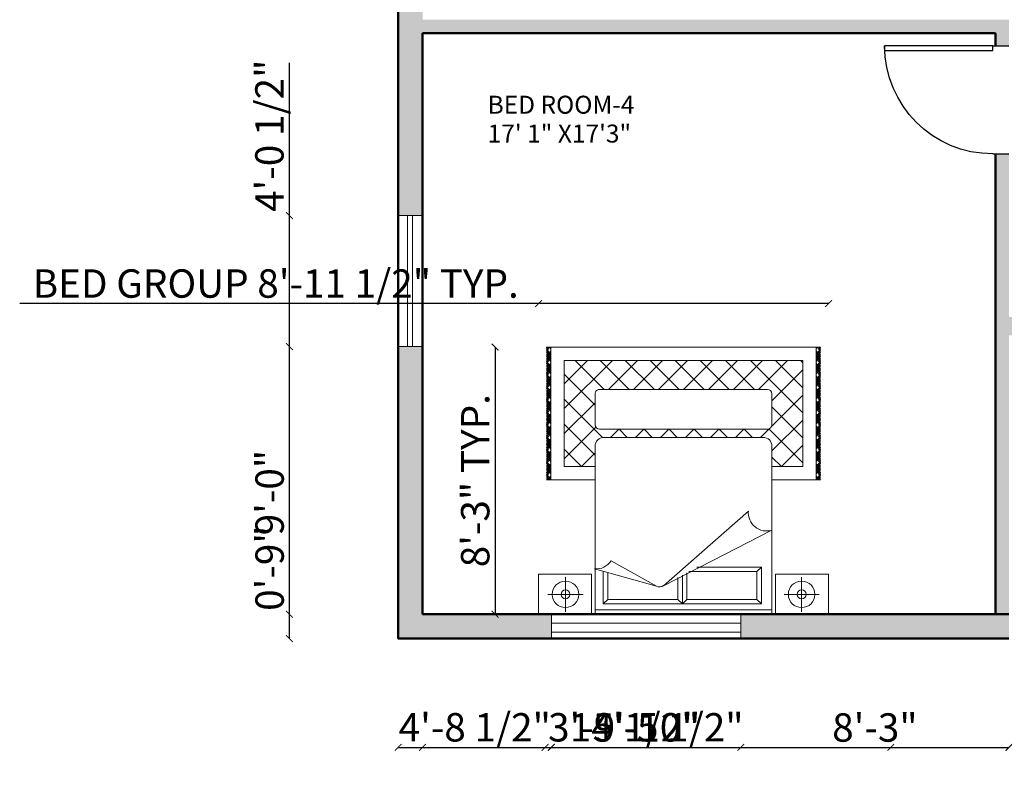
# Model space of a CAD drawing. Units: inches. Extents: x 1549 to 2410, y 1378 to 2139.
# Tile 1 of 6: x 1549 to 1913, y 1378 to 1657. Entities that reach past the tile are written whole.
import ezdxf

# ---------------------------------------------------------------- set-up
doc = ezdxf.new("R2010")
doc.units = ezdxf.units.IN
for name, color, linetype, lineweight in [('A-ANNO-DIMS', 2, 'Continuous', 18), ('A-AREA-IDEN', 7, 'Continuous', 18), ('A-DOOR', 4, 'Continuous', 25), ('A-FURN', 8, 'Continuous', 18), ('A-WALL', 7, 'Continuous', 50), ('WINDOW', 2, 'Continuous', 18)]:
    doc.layers.add(name, color=color, linetype=linetype, lineweight=lineweight)
doc.layers.add('A-WALL-PATT', color=18, linetype='Continuous', lineweight=13, true_color=0x000000)
doc.styles.get("Standard").update_dxf_attribs({"font": 'arial.ttf'})
doc.dimstyles.new('ISO-25', dxfattribs={"dimtxt": 10.5, "dimasz": 2.5, "dimexe": 1.25, "dimexo": 0.625, "dimtad": 1, "dimdec": 0, "dimlunit": 4, "dimtxsty": 'Standard', "dimblk": 'ARCHTICK', "dimcen": 2.5, "dimse1": 1, "dimse2": 1, "dimclrd": 1, "dimclrt": 3, "dimadec": 0, "dimazin": 0, "dimtfac": 1, "dimtdec": 0, "dimtmove": 0, "dimatfit": 3, "dimfxl": 1, "dimarcsym": 0})

# ---------------------------------------------------------------- blocks, each defined once
blk = doc.blocks.new('*U3')
for p, q in [((0, 0), (0, -6)), ((40, 0), (40, -6))]:
    blk.add_line(p, q)
blk.add_lwpolyline([(0, 0), (0, 40), (1.75, 40), (1.75, 0)], close=True)
blk.add_arc((0, 0), 40, 0, 90)
blk = doc.blocks.new('A$C4CB008C5')
for p, q in [((0, 3.019), (0.6, 3.019)), ((0, 2.569), (0, 3.019)), ((0.6, 3.019), (0.6, 2.569)), ((0.64, 1.121), (0.64, 3.021)), ((0.64, 3.021), (2.64, 3.021)), ((2.64, 3.021), (2.64, 1.121)), ((3.279, 3.019), (2.679, 3.019)), ((2.679, 3.019), (2.679, 2.569)), ((3.279, 2.569), (3.279, 3.019)), ((0.304, 2.6), (0.304, 2.992)), ((0.64, 2.971), (2.64, 2.971)), ((0.759, 2.905), (2.547, 2.905)), ((0.759, 2.489), (0.759, 2.905)), ((0.759, 2.905), (0.809, 2.855)), ((1.603, 2.855), (1.653, 2.905)), ((1.653, 2.905), (1.653, 2.579)), ((1.653, 2.905), (1.703, 2.855)), ((2.497, 2.855), (2.547, 2.905)), ((2.547, 2.905), (2.547, 2.54)), ((2.975, 2.6), (2.975, 2.992)), ((0.106, 2.796), (0.503, 2.796)), ((0.809, 2.855), (1.603, 2.855)), ((0.809, 2.539), (0.809, 2.855)), ((1.603, 2.855), (1.603, 2.551)), ((1.703, 2.855), (1.703, 2.607)), ((1.703, 2.855), (2.497, 2.855)), ((2.497, 2.855), (2.497, 2.556)), ((3.174, 2.796), (2.776, 2.796)), ((0.64, 2.071), (1.866, 2.698)), ((0.906, 1.854), (1.866, 2.698)), ((1.946, 2.705), (2.646, 2.507)), ((1.946, 2.705), (2.46, 2.418)), ((0.6, 2.569), (0, 2.569)), ((2.679, 2.569), (3.279, 2.569)), ((0.809, 2.539), (0.759, 2.489)), ((1.49, 2.489), (0.759, 2.489)), ((1.58, 2.539), (0.809, 2.539)), ((0.907, 1.867), (0.919, 1.867)), ((0.09, 1.5), (0.64, 1.5)), ((0.09, 1.491), (0.099, 1.5)), ((0.09, 1.473), (0.116, 1.5)), ((0.09, 1.456), (0.134, 1.5)), ((0.09, 1.474), (0.09, 1.475)), ((0.09, 1.438), (0.126, 1.474)), ((0.117, 1.43), (0.09, 1.457)), ((0.14, 1.46), (0.108, 1.492)), ((0.14, 1.478), (0.118, 1.5)), ((0.14, 1.496), (0.135, 1.5)), ((0.14, 0), (0.14, 1.5)), ((2.64, 1.5), (3.19, 1.5)), ((3.14, 1.496), (3.144, 1.5)), ((3.14, 1.478), (3.162, 1.5)), ((3.14, 1.5), (3.14, 0)), ((3.14, 1.46), (3.171, 1.492)), ((3.19, 1.456), (3.145, 1.5)), ((3.19, 1.438), (3.154, 1.474)), ((3.162, 1.43), (3.19, 1.457)), ((3.19, 1.473), (3.163, 1.5)), ((3.19, 1.491), (3.181, 1.5)), ((3.189, 1.474), (3.19, 1.475)), ((0.14, 1.389), (0.09, 1.439)), ((0.09, 1.42), (0.099, 1.43)), ((0.14, 1.372), (0.09, 1.422)), ((0.09, 1.368), (0.14, 1.417)), ((0.14, 1.354), (0.09, 1.404)), ((0.09, 1.35), (0.14, 1.4)), ((0.14, 1.336), (0.09, 1.386)), ((0.09, 1.332), (0.14, 1.382)), ((0.09, 1.314), (0.14, 1.364)), ((0.14, 1.319), (0.108, 1.35)), ((0.117, 1.412), (0.14, 1.435)), ((0.14, 1.442), (0.135, 1.448)), ((0.29, 1.108), (0.532, 1.35)), ((0.29, 0.15), (0.29, 1.35)), ((0.29, 1.35), (0.64, 1.35)), ((0.64, 1.243), (0.533, 1.35)), ((2.64, 1.195), (2.795, 1.35)), ((2.64, 1.35), (2.99, 1.35)), ((2.99, 1.156), (2.795, 1.35)), ((2.99, 1.35), (2.99, 0.15)), ((3.14, 1.442), (3.145, 1.448)), ((3.14, 1.389), (3.19, 1.439)), ((3.162, 1.412), (3.14, 1.435)), ((3.14, 1.372), (3.19, 1.422)), ((3.189, 1.368), (3.14, 1.417)), ((3.14, 1.354), (3.19, 1.404)), ((3.19, 1.35), (3.14, 1.4)), ((3.14, 1.336), (3.19, 1.386)), ((3.19, 1.332), (3.14, 1.382)), ((3.19, 1.314), (3.14, 1.364)), ((3.14, 1.319), (3.171, 1.35)), ((3.19, 1.42), (3.18, 1.43)), ((0.09, 1.297), (0.126, 1.333)), ((0.09, 1.333), (0.09, 1.333)), ((0.117, 1.288), (0.09, 1.316)), ((0.14, 1.248), (0.09, 1.298)), ((0.09, 1.279), (0.099, 1.288)), ((0.14, 1.23), (0.09, 1.28)), ((0.09, 1.227), (0.14, 1.276)), ((0.14, 1.213), (0.09, 1.263)), ((0.09, 1.208), (0.14, 1.258)), ((0.14, 1.195), (0.09, 1.245)), ((0.09, 1.19), (0.14, 1.24)), ((0.117, 1.271), (0.14, 1.294)), ((0.14, 1.301), (0.135, 1.306)), ((0.674, 0.926), (0.29, 1.31)), ((2.632, 0.904), (2.99, 1.262)), ((3.14, 1.301), (3.145, 1.306)), ((3.14, 1.248), (3.19, 1.298)), ((3.162, 1.271), (3.14, 1.294)), ((3.14, 1.23), (3.19, 1.28)), ((3.189, 1.227), (3.14, 1.276)), ((3.14, 1.213), (3.19, 1.263)), ((3.19, 1.208), (3.14, 1.258)), ((3.14, 1.195), (3.19, 1.245)), ((3.19, 1.19), (3.14, 1.24)), ((3.19, 1.297), (3.154, 1.333)), ((3.162, 1.288), (3.19, 1.316)), ((3.19, 1.279), (3.18, 1.288)), ((3.189, 1.333), (3.19, 1.333)), ((0.09, 1.173), (0.14, 1.223)), ((0.09, 1.191), (0.09, 1.192)), ((0.09, 1.155), (0.126, 1.191)), ((0.117, 1.147), (0.09, 1.174)), ((0.14, 1.107), (0.09, 1.157)), ((0.09, 1.137), (0.099, 1.147)), ((0.14, 1.089), (0.09, 1.139)), ((0.09, 1.085), (0.14, 1.134)), ((0.14, 1.071), (0.09, 1.121)), ((0.09, 1.067), (0.14, 1.117)), ((0.14, 1.177), (0.108, 1.209)), ((0.117, 1.129), (0.14, 1.152)), ((0.14, 1.16), (0.135, 1.165)), ((0.29, 0.825), (0.64, 1.175)), ((2.99, 0.873), (2.64, 1.223)), ((3.19, 1.173), (3.14, 1.223)), ((3.14, 1.177), (3.171, 1.209)), ((3.14, 1.16), (3.145, 1.165)), ((3.14, 1.107), (3.19, 1.157)), ((3.162, 1.129), (3.14, 1.152)), ((3.14, 1.089), (3.19, 1.139)), ((3.189, 1.085), (3.14, 1.134)), ((3.14, 1.071), (3.19, 1.121)), ((3.19, 1.067), (3.14, 1.117)), ((3.19, 1.155), (3.154, 1.191)), ((3.162, 1.147), (3.19, 1.174)), ((3.19, 1.137), (3.18, 1.147)), ((3.189, 1.191), (3.19, 1.192)), ((0.14, 1.054), (0.09, 1.104)), ((0.09, 1.049), (0.14, 1.099)), ((0.09, 1.031), (0.14, 1.081)), ((0.09, 1.05), (0.09, 1.051)), ((0.09, 1.014), (0.126, 1.05)), ((0.117, 1.006), (0.09, 1.033)), ((0.14, 0.965), (0.09, 1.015)), ((0.09, 0.996), (0.099, 1.006)), ((0.14, 1.036), (0.108, 1.067)), ((0.117, 0.988), (0.14, 1.011)), ((0.14, 1.018), (0.135, 1.023)), ((0.64, 0.677), (0.29, 1.027)), ((0.673, 0.925), (0.769, 1.021)), ((2.54, 1.021), (0.74, 1.021)), ((0.955, 0.928), (0.861, 1.021)), ((0.959, 0.928), (1.052, 1.021)), ((1.238, 0.928), (1.144, 1.021)), ((1.241, 0.928), (1.335, 1.021)), ((1.52, 0.928), (1.427, 1.021)), ((1.524, 0.928), (1.618, 1.021)), ((1.803, 0.928), (1.71, 1.021)), ((1.807, 0.928), (1.9, 1.021)), ((2.086, 0.928), (1.993, 1.021)), ((2.09, 0.928), (2.183, 1.021)), ((2.369, 0.928), (2.276, 1.021)), ((2.373, 0.928), (2.466, 1.021)), ((2.99, 0.59), (2.557, 1.023)), ((3.14, 1.054), (3.19, 1.104)), ((3.19, 1.049), (3.14, 1.099)), ((3.19, 1.031), (3.14, 1.081)), ((3.14, 1.036), (3.171, 1.067)), ((3.14, 1.018), (3.145, 1.023)), ((3.14, 0.965), (3.19, 1.015)), ((3.162, 0.988), (3.14, 1.011)), ((3.19, 1.014), (3.154, 1.05)), ((3.162, 1.006), (3.19, 1.033)), ((3.19, 0.996), (3.18, 1.006)), ((3.189, 1.05), (3.19, 1.051)), ((0.14, 0.948), (0.09, 0.998)), ((0.09, 0.944), (0.14, 0.993)), ((0.14, 0.93), (0.09, 0.98)), ((0.09, 0.925), (0.14, 0.975)), ((0.14, 0.912), (0.09, 0.962)), ((0.09, 0.908), (0.14, 0.958)), ((0.09, 0.89), (0.14, 0.94)), ((0.09, 0.908), (0.09, 0.909)), ((0.09, 0.872), (0.126, 0.908)), ((0.117, 0.864), (0.09, 0.891)), ((0.14, 0.894), (0.108, 0.926)), ((0.29, 0.542), (0.643, 0.895)), ((0.69, 0.928), (2.59, 0.928)), ((2.64, 0.629), (2.99, 0.979)), ((3.14, 0.948), (3.19, 0.998)), ((3.189, 0.944), (3.14, 0.993)), ((3.14, 0.93), (3.19, 0.98)), ((3.19, 0.925), (3.14, 0.975)), ((3.14, 0.912), (3.19, 0.962)), ((3.19, 0.908), (3.14, 0.958)), ((3.19, 0.89), (3.14, 0.94)), ((3.14, 0.894), (3.171, 0.926)), ((3.19, 0.872), (3.154, 0.908)), ((3.162, 0.864), (3.19, 0.891)), ((3.189, 0.908), (3.19, 0.909)), ((0.14, 0.824), (0.09, 0.874)), ((0.09, 0.855), (0.099, 0.864)), ((0.14, 0.806), (0.09, 0.856)), ((0.09, 0.802), (0.14, 0.852)), ((0.14, 0.788), (0.09, 0.838)), ((0.09, 0.784), (0.14, 0.834)), ((0.14, 0.771), (0.09, 0.821)), ((0.09, 0.766), (0.14, 0.816)), ((0.09, 0.749), (0.14, 0.799)), ((0.14, 0.753), (0.108, 0.785)), ((0.117, 0.847), (0.14, 0.869)), ((0.14, 0.877), (0.135, 0.882)), ((0.64, 0.878), (0.64, 0.528)), ((2.64, 0.878), (2.64, 0.528)), ((3.14, 0.877), (3.145, 0.882)), ((3.14, 0.824), (3.19, 0.874)), ((3.162, 0.847), (3.14, 0.869)), ((3.14, 0.806), (3.19, 0.856)), ((3.189, 0.802), (3.14, 0.852)), ((3.14, 0.788), (3.19, 0.838)), ((3.19, 0.784), (3.14, 0.834)), ((3.14, 0.771), (3.19, 0.821)), ((3.19, 0.766), (3.14, 0.816)), ((3.19, 0.749), (3.14, 0.799)), ((3.14, 0.753), (3.171, 0.785)), ((3.19, 0.855), (3.18, 0.864)), ((0.09, 0.767), (0.09, 0.768)), ((0.09, 0.731), (0.126, 0.767)), ((0.117, 0.723), (0.09, 0.75)), ((0.14, 0.682), (0.09, 0.732)), ((0.09, 0.713), (0.099, 0.723)), ((0.14, 0.665), (0.09, 0.715)), ((0.09, 0.661), (0.14, 0.71)), ((0.14, 0.647), (0.09, 0.697)), ((0.09, 0.642), (0.14, 0.692)), ((0.14, 0.629), (0.09, 0.679)), ((0.09, 0.625), (0.14, 0.675)), ((0.117, 0.705), (0.14, 0.728)), ((0.14, 0.735), (0.135, 0.74)), ((0.884, 0.15), (0.29, 0.744)), ((2.443, 0.15), (2.99, 0.696)), ((3.14, 0.735), (3.145, 0.74)), ((3.14, 0.682), (3.19, 0.732)), ((3.162, 0.705), (3.14, 0.728)), ((3.14, 0.665), (3.19, 0.715)), ((3.189, 0.661), (3.14, 0.71)), ((3.14, 0.647), (3.19, 0.697)), ((3.19, 0.642), (3.14, 0.692)), ((3.14, 0.629), (3.19, 0.679)), ((3.19, 0.625), (3.14, 0.675)), ((3.19, 0.731), (3.154, 0.767)), ((3.162, 0.723), (3.19, 0.75)), ((3.19, 0.713), (3.18, 0.723)), ((3.189, 0.767), (3.19, 0.768)), ((0.09, 0.607), (0.14, 0.657)), ((0.09, 0.589), (0.126, 0.626)), ((0.09, 0.626), (0.09, 0.626)), ((0.117, 0.581), (0.09, 0.609)), ((0.14, 0.541), (0.09, 0.591)), ((0.09, 0.572), (0.099, 0.581)), ((0.14, 0.523), (0.09, 0.573)), ((0.09, 0.519), (0.14, 0.569)), ((0.14, 0.612), (0.108, 0.643)), ((0.117, 0.564), (0.14, 0.586)), ((0.14, 0.594), (0.135, 0.599)), ((0.29, 0.259), (0.64, 0.609)), ((2.99, 0.307), (2.64, 0.657)), ((3.19, 0.607), (3.14, 0.657)), ((3.14, 0.612), (3.171, 0.643)), ((3.14, 0.594), (3.145, 0.599)), ((3.14, 0.541), (3.19, 0.591)), ((3.162, 0.564), (3.14, 0.586)), ((3.14, 0.523), (3.19, 0.573)), ((3.189, 0.519), (3.14, 0.569)), ((3.19, 0.589), (3.154, 0.626)), ((3.162, 0.581), (3.19, 0.609)), ((3.19, 0.572), (3.18, 0.581)), ((3.189, 0.626), (3.19, 0.626)), ((0.14, 0.506), (0.09, 0.556)), ((0.09, 0.501), (0.14, 0.551)), ((0.14, 0.488), (0.09, 0.538)), ((0.09, 0.483), (0.14, 0.533)), ((0.09, 0.466), (0.14, 0.516)), ((0.09, 0.484), (0.09, 0.485)), ((0.09, 0.448), (0.126, 0.484)), ((0.117, 0.44), (0.09, 0.467)), ((0.14, 0.399), (0.09, 0.449)), ((0.14, 0.47), (0.108, 0.502)), ((0.14, 0.453), (0.135, 0.458)), ((0.601, 0.15), (0.29, 0.462)), ((0.463, 0.15), (0.791, 0.478)), ((0.69, 0.478), (2.59, 0.478)), ((0.746, 0.15), (1.074, 0.478)), ((1.167, 0.15), (0.839, 0.478)), ((1.029, 0.15), (1.357, 0.478)), ((1.45, 0.15), (1.122, 0.478)), ((1.312, 0.15), (1.64, 0.478)), ((1.733, 0.15), (1.405, 0.478)), ((1.595, 0.15), (1.923, 0.478)), ((2.016, 0.15), (1.688, 0.478)), ((1.878, 0.15), (2.206, 0.478)), ((2.298, 0.15), (1.97, 0.478)), ((2.16, 0.15), (2.488, 0.478)), ((2.581, 0.15), (2.253, 0.478)), ((2.864, 0.15), (2.536, 0.478)), ((3.14, 0.506), (3.19, 0.556)), ((3.19, 0.501), (3.14, 0.551)), ((3.14, 0.488), (3.19, 0.538)), ((3.19, 0.483), (3.14, 0.533)), ((3.19, 0.466), (3.14, 0.516)), ((3.14, 0.47), (3.171, 0.502)), ((3.14, 0.453), (3.145, 0.458)), ((3.14, 0.399), (3.19, 0.449)), ((3.19, 0.448), (3.154, 0.484)), ((3.162, 0.44), (3.19, 0.467)), ((3.189, 0.484), (3.19, 0.485)), ((0.09, 0.43), (0.099, 0.44)), ((0.14, 0.382), (0.09, 0.432)), ((0.09, 0.378), (0.14, 0.427)), ((0.14, 0.364), (0.09, 0.414)), ((0.09, 0.36), (0.14, 0.41)), ((0.14, 0.346), (0.09, 0.396)), ((0.09, 0.342), (0.14, 0.392)), ((0.09, 0.324), (0.14, 0.374)), ((0.09, 0.307), (0.126, 0.343)), ((0.09, 0.343), (0.09, 0.343)), ((0.14, 0.329), (0.108, 0.36)), ((0.117, 0.422), (0.14, 0.445)), ((2.726, 0.15), (2.99, 0.414)), ((3.162, 0.422), (3.14, 0.445)), ((3.14, 0.382), (3.19, 0.432)), ((3.189, 0.378), (3.14, 0.427)), ((3.14, 0.364), (3.19, 0.414)), ((3.19, 0.36), (3.14, 0.41)), ((3.14, 0.346), (3.19, 0.396)), ((3.19, 0.342), (3.14, 0.392)), ((3.19, 0.324), (3.14, 0.374)), ((3.14, 0.329), (3.171, 0.36)), ((3.19, 0.307), (3.154, 0.343)), ((3.19, 0.43), (3.18, 0.44)), ((3.189, 0.343), (3.19, 0.343)), ((0.117, 0.299), (0.09, 0.326)), ((0.14, 0.258), (0.09, 0.308)), ((0.09, 0.289), (0.099, 0.299)), ((0.14, 0.24), (0.09, 0.29)), ((0.09, 0.237), (0.14, 0.286)), ((0.14, 0.223), (0.09, 0.273)), ((0.09, 0.218), (0.14, 0.268)), ((0.14, 0.205), (0.09, 0.255)), ((0.09, 0.201), (0.14, 0.251)), ((0.09, 0.183), (0.14, 0.233)), ((0.117, 0.281), (0.14, 0.304)), ((0.14, 0.311), (0.135, 0.316)), ((3.14, 0.311), (3.145, 0.316)), ((3.14, 0.258), (3.19, 0.308)), ((3.162, 0.281), (3.14, 0.304)), ((3.14, 0.24), (3.19, 0.29)), ((3.189, 0.237), (3.14, 0.286)), ((3.14, 0.223), (3.19, 0.273)), ((3.19, 0.218), (3.14, 0.268)), ((3.14, 0.205), (3.19, 0.255)), ((3.19, 0.201), (3.14, 0.251)), ((3.19, 0.183), (3.14, 0.233)), ((3.162, 0.299), (3.19, 0.326)), ((3.19, 0.289), (3.18, 0.299)), ((0.09, 0.201), (0.09, 0.202)), ((0.09, 0.165), (0.126, 0.201)), ((0.117, 0.157), (0.09, 0.184)), ((0.14, 0.117), (0.09, 0.167)), ((0.09, 0.148), (0.099, 0.157)), ((0.14, 0.099), (0.09, 0.149)), ((0.09, 0.095), (0.14, 0.144)), ((0.14, 0.081), (0.09, 0.131)), ((0.09, 0.077), (0.14, 0.127)), ((0.14, 0.064), (0.09, 0.114)), ((0.14, 0.187), (0.108, 0.219)), ((0.117, 0.139), (0.14, 0.162)), ((0.14, 0.17), (0.135, 0.175)), ((0.318, 0.15), (0.29, 0.179)), ((2.99, 0.15), (0.29, 0.15)), ((3.14, 0.187), (3.171, 0.219)), ((3.14, 0.17), (3.145, 0.175)), ((3.14, 0.117), (3.19, 0.167)), ((3.162, 0.139), (3.14, 0.162)), ((3.14, 0.099), (3.19, 0.149)), ((3.189, 0.095), (3.14, 0.144)), ((3.14, 0.081), (3.19, 0.131)), ((3.19, 0.077), (3.14, 0.127)), ((3.14, 0.064), (3.19, 0.114)), ((3.19, 0.165), (3.154, 0.201)), ((3.162, 0.157), (3.19, 0.184)), ((3.19, 0.148), (3.18, 0.157)), ((3.189, 0.201), (3.19, 0.202)), ((0.09, 0.059), (0.14, 0.109)), ((0.09, 0.041), (0.14, 0.091)), ((0.09, 0.06), (0.09, 0.061)), ((0.09, 0.024), (0.126, 0.06)), ((0.117, 0.016), (0.09, 0.043)), ((0.115, 0), (0.09, 0.025)), ((0.09, 0.006), (0.099, 0.016)), ((0.097, 0), (0.09, 0.008)), ((0.14, 0.046), (0.108, 0.078)), ((0.119, 0), (0.14, 0.021)), ((0.14, 0.028), (0.135, 0.033)), ((0.137, 0), (0.14, 0.003)), ((3.19, 0.059), (3.14, 0.109)), ((3.19, 0.041), (3.14, 0.091)), ((3.14, 0.046), (3.171, 0.078)), ((3.14, 0.028), (3.145, 0.033)), ((3.16, 0), (3.14, 0.021)), ((3.143, 0), (3.14, 0.003)), ((3.19, 0.024), (3.154, 0.06)), ((3.162, 0.016), (3.19, 0.043)), ((3.164, 0), (3.19, 0.025)), ((3.19, 0.006), (3.18, 0.016)), ((3.182, 0), (3.19, 0.008)), ((3.189, 0.06), (3.19, 0.061)), ((0.09, 0), (3.19, 0))]:
    blk.add_line(p, q)
for centre, radius in [((0.304, 2.796), 0.15), ((2.975, 2.796), 0.15), ((0.304, 2.796), 0.05), ((2.975, 2.796), 0.05)]:
    blk.add_circle(centre, radius)
for centre, radius, start, end in [((1.915, 2.61), 0.1, 71.7215, 119.0799), ((2.626, 2.31), 0.198, 84.1725, 146.9889), ((0.7, 1.873), 0.207, 354.6422, 106.9775), ((0.74, 1.121), 0.1, 180, 270), ((2.54, 1.121), 0.1, 270, 0), ((0.69, 0.878), 0.05, 90, 180), ((2.59, 0.878), 0.05, 0, 90), ((0.69, 0.528), 0.05, 180, 270), ((2.59, 0.528), 0.05, 270, 0)]:
    blk.add_arc(centre, radius, start, end)
blk = doc.blocks.new('_ArchTick')
at = {"color": 0, "linetype": 'ByBlock', "const_width": 0.15}
blk.add_lwpolyline([(-0.5, -0.5), (0.5, 0.5)], dxfattribs=at)
blk = doc.blocks.new('*D15')
at = {"layer": 'A-ANNO-DIMS', "color": 1, "lineweight": -2, "transparency": 16777216}
for p, q in [((1740.55, 1551.97), (1548.54, 1551.97)), ((1847.85, 1551.97), (1740.55, 1551.97))]:
    blk.add_line(p, q, dxfattribs=at)
at = {"layer": 'Defpoints', "color": 0, "transparency": 16777216}
for p in [(1740.55, 1551.97), (1740.55, 1535.87), (1847.85, 1535.87)]:
    blk.add_point(p, dxfattribs=at)
at = {"layer": 'A-ANNO-DIMS', "color": 1, "lineweight": -2, "transparency": 16777216, "xscale": 2.5, "yscale": 2.5, "zscale": 2.5, "rotation": 180}
blk.add_blockref('_ArchTick', (1740.55, 1551.97), dxfattribs=at)
at = {"layer": 'A-ANNO-DIMS', "color": 1, "lineweight": -2, "transparency": 16777216, "xscale": 2.5, "yscale": 2.5, "zscale": 2.5}
blk.add_blockref('_ArchTick', (1847.85, 1551.97), dxfattribs=at)
at = {"layer": 'A-ANNO-DIMS', "color": 3, "transparency": 16777216, "insert": (1643.29, 1558.03), "char_height": 10.5, "attachment_point": 5}
blk.add_mtext('BED GROUP 8\'-11 1/2" TYP.', dxfattribs=at)
blk = doc.blocks.new('*D16')
at = {"layer": 'A-ANNO-DIMS', "color": 1, "lineweight": -2, "transparency": 16777216}
blk.add_line((1724.45, 1535.87), (1724.45, 1437.01), dxfattribs=at)
at = {"layer": 'Defpoints', "color": 0, "transparency": 16777216}
for p in [(1740.55, 1535.87), (1724.45, 1437.01), (1740.55, 1437.01)]:
    blk.add_point(p, dxfattribs=at)
at = {"layer": 'A-ANNO-DIMS', "color": 1, "lineweight": -2, "transparency": 16777216, "xscale": 2.5, "yscale": 2.5, "zscale": 2.5}
for p, rotation in [((1724.45, 1535.87), 90), ((1724.45, 1437.01), 270)]:
    blk.add_blockref('_ArchTick', p, dxfattribs=dict(at, rotation=rotation))
at = {"layer": 'A-ANNO-DIMS', "color": 3, "transparency": 16777216, "insert": (1718.46, 1486.44), "char_height": 10.5, "attachment_point": 5, "rotation": 90}
blk.add_mtext('8\'-3" TYP.', dxfattribs=at)
blk = doc.blocks.new('*D27')
at = {"layer": 'A-ANNO-DIMS', "color": 1, "lineweight": -2, "transparency": 16777216}
blk.add_line((1688.62, 1387.76), (1745.28, 1387.76), dxfattribs=at)
at = {"layer": 'Defpoints', "color": 0, "transparency": 16777216}
for p in [(1688.62, 1428.01), (1745.28, 1428.01), (1745.28, 1387.76)]:
    blk.add_point(p, dxfattribs=at)
at = {"layer": 'A-ANNO-DIMS', "color": 1, "lineweight": -2, "transparency": 16777216, "xscale": 2.5, "yscale": 2.5, "zscale": 2.5, "rotation": 180}
blk.add_blockref('_ArchTick', (1688.62, 1387.76), dxfattribs=at)
at = {"layer": 'A-ANNO-DIMS', "color": 1, "lineweight": -2, "transparency": 16777216, "xscale": 2.5, "yscale": 2.5, "zscale": 2.5}
blk.add_blockref('_ArchTick', (1745.28, 1387.76), dxfattribs=at)
at = {"layer": 'A-ANNO-DIMS', "color": 3, "transparency": 16777216, "insert": (1716.95, 1393.82), "char_height": 10.5, "attachment_point": 5}
blk.add_mtext('4\'-8 1/2"', dxfattribs=at)
blk = doc.blocks.new('*D28')
at = {"layer": 'A-ANNO-DIMS', "color": 1, "lineweight": -2, "transparency": 16777216}
blk.add_line((1745.28, 1387.76), (1815.42, 1387.76), dxfattribs=at)
at = {"layer": 'Defpoints', "color": 0, "transparency": 16777216}
for p in [(1745.28, 1428.01), (1815.42, 1428.01), (1815.42, 1387.76)]:
    blk.add_point(p, dxfattribs=at)
at = {"layer": 'A-ANNO-DIMS', "color": 1, "lineweight": -2, "transparency": 16777216, "xscale": 2.5, "yscale": 2.5, "zscale": 2.5, "rotation": 180}
blk.add_blockref('_ArchTick', (1745.28, 1387.76), dxfattribs=at)
at = {"layer": 'A-ANNO-DIMS', "color": 1, "lineweight": -2, "transparency": 16777216, "xscale": 2.5, "yscale": 2.5, "zscale": 2.5}
blk.add_blockref('_ArchTick', (1815.42, 1387.76), dxfattribs=at)
at = {"layer": 'A-ANNO-DIMS', "color": 3, "transparency": 16777216, "insert": (1780.35, 1393.75), "char_height": 10.5, "attachment_point": 5}
blk.add_mtext('5\'-10"', dxfattribs=at)
blk = doc.blocks.new('*D29')
at = {"layer": 'A-ANNO-DIMS', "color": 1, "lineweight": -2, "transparency": 16777216}
blk.add_line((1815.42, 1387.76), (1914.62, 1387.76), dxfattribs=at)
at = {"layer": 'Defpoints', "color": 0, "transparency": 16777216}
for p in [(1815.42, 1428.01), (1914.62, 1428.01), (1914.62, 1387.76)]:
    blk.add_point(p, dxfattribs=at)
at = {"layer": 'A-ANNO-DIMS', "color": 1, "lineweight": -2, "transparency": 16777216, "xscale": 2.5, "yscale": 2.5, "zscale": 2.5, "rotation": 180}
blk.add_blockref('_ArchTick', (1815.42, 1387.76), dxfattribs=at)
at = {"layer": 'A-ANNO-DIMS', "color": 1, "lineweight": -2, "transparency": 16777216, "xscale": 2.5, "yscale": 2.5, "zscale": 2.5}
blk.add_blockref('_ArchTick', (1914.62, 1387.76), dxfattribs=at)
at = {"layer": 'A-ANNO-DIMS', "color": 3, "transparency": 16777216, "insert": (1865.02, 1393.75), "char_height": 10.5, "attachment_point": 5}
blk.add_mtext('8\'-3"', dxfattribs=at)
blk = doc.blocks.new('*D35')
at = {"layer": 'A-ANNO-DIMS', "color": 1, "lineweight": -2, "transparency": 16777216}
blk.add_line((1648.37, 1428.01), (1648.37, 1536.06), dxfattribs=at)
at = {"layer": 'Defpoints', "color": 0, "transparency": 16777216}
for p in [(1648.37, 1536.06), (1688.62, 1536.06), (1688.62, 1428.01)]:
    blk.add_point(p, dxfattribs=at)
at = {"layer": 'A-ANNO-DIMS', "color": 1, "lineweight": -2, "transparency": 16777216, "xscale": 2.5, "yscale": 2.5, "zscale": 2.5}
for p, rotation in [((1648.37, 1536.06), 90), ((1648.37, 1428.01), 270)]:
    blk.add_blockref('_ArchTick', p, dxfattribs=dict(at, rotation=rotation))
at = {"layer": 'A-ANNO-DIMS', "color": 3, "transparency": 16777216, "insert": (1642.38, 1482.04), "char_height": 10.5, "attachment_point": 5, "rotation": 90}
blk.add_mtext('9\'-0"', dxfattribs=at)
blk = doc.blocks.new('*D36')
at = {"layer": 'A-ANNO-DIMS', "color": 1, "lineweight": -2, "transparency": 16777216}
for p, q in [((1648.37, 1584.55), (1648.37, 1641.1)), ((1648.37, 1536.06), (1648.37, 1584.55))]:
    blk.add_line(p, q, dxfattribs=at)
at = {"layer": 'Defpoints', "color": 0, "transparency": 16777216}
for p in [(1648.37, 1584.55), (1688.62, 1584.55), (1688.62, 1536.06)]:
    blk.add_point(p, dxfattribs=at)
at = {"layer": 'A-ANNO-DIMS', "color": 1, "lineweight": -2, "transparency": 16777216, "xscale": 2.5, "yscale": 2.5, "zscale": 2.5}
for p, rotation in [((1648.37, 1584.55), 90), ((1648.37, 1536.06), 270)]:
    blk.add_blockref('_ArchTick', p, dxfattribs=dict(at, rotation=rotation))
at = {"layer": 'A-ANNO-DIMS', "color": 3, "transparency": 16777216, "insert": (1642.31, 1614.08), "char_height": 10.5, "attachment_point": 5, "rotation": 90}
blk.add_mtext('4\'-0 1/2"', dxfattribs=at)
blk = doc.blocks.new('*D55')
at = {"layer": 'A-ANNO-DIMS', "color": 1, "lineweight": -2, "transparency": 16777216}
for p, q in [((1648.37, 1437.01), (1648.37, 1468.68)), ((1648.37, 1428.01), (1648.37, 1437.01))]:
    blk.add_line(p, q, dxfattribs=at)
at = {"layer": 'Defpoints', "color": 0, "transparency": 16777216}
for p in [(1648.37, 1437.01), (1697.62, 1437.01), (1688.62, 1428.01)]:
    blk.add_point(p, dxfattribs=at)
at = {"layer": 'A-ANNO-DIMS', "color": 1, "lineweight": -2, "transparency": 16777216, "xscale": 2.5, "yscale": 2.5, "zscale": 2.5}
for p, rotation in [((1648.37, 1437.01), 90), ((1648.37, 1428.01), 270)]:
    blk.add_blockref('_ArchTick', p, dxfattribs=dict(at, rotation=rotation))
at = {"layer": 'A-ANNO-DIMS', "color": 3, "transparency": 16777216, "insert": (1642.38, 1454.1), "char_height": 10.5, "attachment_point": 5, "rotation": 90}
blk.add_mtext('0\'-9"', dxfattribs=at)
blk = doc.blocks.new('*D60')
at = {"layer": 'A-ANNO-DIMS', "color": 1, "lineweight": -2, "transparency": 16777216}
blk.add_line((2400.7, 1657.01), (2400.7, 1709.88), dxfattribs=at)
at = {"layer": 'Defpoints', "color": 0, "transparency": 16777216}
for p in [(1870.93, 1709.88), (2400.7, 1709.88), (1870.93, 1657.01)]:
    blk.add_point(p, dxfattribs=at)
at = {"layer": 'A-ANNO-DIMS', "color": 1, "lineweight": -2, "transparency": 16777216, "xscale": 2.5, "yscale": 2.5, "zscale": 2.5}
for p, rotation in [((2400.7, 1709.88), 90), ((2400.7, 1657.01), 270)]:
    blk.add_blockref('_ArchTick', p, dxfattribs=dict(at, rotation=rotation))
at = {"layer": 'A-ANNO-DIMS', "color": 3, "transparency": 16777216, "insert": (2394.74, 1683.45), "char_height": 10.5, "attachment_point": 5, "rotation": 90}
blk.add_mtext('4\'-5"', dxfattribs=at)
blk = doc.blocks.new('*D61')
at = {"layer": 'A-ANNO-DIMS', "color": 1, "lineweight": -2, "transparency": 16777216}
for p, q in [((1697.62, 1387.76), (1742.95, 1387.76)), ((1742.95, 1387.76), (1799.07, 1387.76))]:
    blk.add_line(p, q, dxfattribs=at)
at = {"layer": 'Defpoints', "color": 0, "transparency": 16777216}
for p in [(1697.62, 1764.95), (1742.95, 1764.95), (1742.95, 1387.76)]:
    blk.add_point(p, dxfattribs=at)
at = {"layer": 'A-ANNO-DIMS', "color": 1, "lineweight": -2, "transparency": 16777216, "xscale": 2.5, "yscale": 2.5, "zscale": 2.5, "rotation": 180}
blk.add_blockref('_ArchTick', (1697.62, 1387.76), dxfattribs=at)
at = {"layer": 'A-ANNO-DIMS', "color": 1, "lineweight": -2, "transparency": 16777216, "xscale": 2.5, "yscale": 2.5, "zscale": 2.5}
blk.add_blockref('_ArchTick', (1742.95, 1387.76), dxfattribs=at)
at = {"layer": 'A-ANNO-DIMS', "color": 3, "transparency": 16777216, "insert": (1772.26, 1393.82), "char_height": 10.5, "attachment_point": 5}
blk.add_mtext('3\'-9 1/2"', dxfattribs=at)
blk = doc.blocks.new('*D62')
at = {"layer": 'A-ANNO-DIMS', "color": 1, "lineweight": -2, "transparency": 16777216}
blk.add_line((1697.62, 1387.76), (1870.93, 1387.76), dxfattribs=at)
at = {"layer": 'Defpoints', "color": 0, "transparency": 16777216}
for p in [(1697.62, 1657.01), (1870.93, 1657.01), (1870.93, 1387.76)]:
    blk.add_point(p, dxfattribs=at)
at = {"layer": 'A-ANNO-DIMS', "color": 1, "lineweight": -2, "transparency": 16777216, "xscale": 2.5, "yscale": 2.5, "zscale": 2.5, "rotation": 180}
blk.add_blockref('_ArchTick', (1697.62, 1387.76), dxfattribs=at)
at = {"layer": 'A-ANNO-DIMS', "color": 1, "lineweight": -2, "transparency": 16777216, "xscale": 2.5, "yscale": 2.5, "zscale": 2.5}
blk.add_blockref('_ArchTick', (1870.93, 1387.76), dxfattribs=at)
at = {"layer": 'A-ANNO-DIMS', "color": 3, "transparency": 16777216, "insert": (1784.28, 1393.82), "char_height": 10.5, "attachment_point": 5}
blk.add_mtext('14\'-5 1/2"', dxfattribs=at)

msp = doc.modelspace()

# ---------------------------------------------------------------- hatches: boundary and pattern name
at = {"layer": 'A-WALL-PATT'}
h = msp.add_hatch(color=256, dxfattribs=at)
h.dxf.hatch_style = 1
h.paths.add_polyline_path([(1760, 2069.01), (1688.62, 2069.01), (1688.62, 2003.68), (1697.62, 2003.68), (1697.62, 2060.01), (1760, 2060.01)])
h.paths.add_polyline_path([(2309.62, 2069.01), (1807.68, 2069.01), (1807.68, 2060.01), (1909.62, 2060.01), (1909.62, 2040.27), (1914.62, 2040.27), (1914.62, 2060.01), (2082.62, 2060.01), (2082.62, 2043.41), (2087.62, 2043.41), (2087.62, 2060.01), (2300.62, 2060.01), (2300.62, 2006.22), (2309.62, 2006.22)])
h.paths.add_polyline_path([(1914.62, 1607.36), (1909.62, 1607.36), (1909.62, 1437.01), (1914.62, 1437.01)])
h.paths.add_polyline_path([(1697.62, 1536.06), (1688.62, 1536.06), (1688.62, 1428.01), (1745.28, 1428.01), (1745.28, 1437.01), (1697.62, 1437.01)])
h.paths.add_polyline_path([(2130.61, 1437.01), (2082.62, 1437.01), (2082.62, 1428.01), (2130.61, 1428.01)])
h.paths.add_polyline_path([(2309.62, 1544.51), (2302.25, 1544.51), (2302.25, 1524.81), (2300.62, 1524.81), (2300.62, 1523.51), (2302.17, 1523.51), (2302.17, 1503.88), (2300.62, 1503.88), (2300.62, 1437.01), (2193.34, 1437.01), (2193.34, 1428.01), (2309.62, 1428.01)])
h.paths.add_polyline_path([(2309.62, 1708.66), (2300.62, 1708.66), (2300.62, 1657.01), (2293.7, 1657.01), (2293.7, 1652.01), (2300.62, 1652.01), (2300.62, 1611.18), (2302.17, 1611.18), (2302.17, 1597.64), (2309.62, 1597.64)])
h.paths.add_polyline_path([(2309.62, 1777.38), (2300.62, 1777.38), (2300.62, 1737.9), (2309.62, 1737.9)])
h.paths.add_polyline_path([(2300.62, 1757.01), (2168.62, 1757.01), (2168.62, 1795.96), (2163.62, 1795.96), (2163.62, 1657.01), (2082.62, 1657.01), (2082.62, 1641.99), (2087.62, 1641.99), (2087.62, 1652.01), (2253.7, 1652.01), (2253.7, 1657.01), (2168.62, 1657.01), (2168.62, 1752.01), (2300.62, 1752.01)])
h.paths.add_polyline_path([(2309.62, 1957.79), (2300.62, 1957.79), (2300.62, 1935.33), (2300.62, 1824.93), (2309.62, 1824.93)])
h.paths.add_polyline_path([(2300.62, 1849.01), (2137.17, 1849.01), (2137.17, 1844.01), (2163.62, 1844.01), (2163.62, 1835.96), (2168.62, 1835.96), (2168.62, 1844.01), (2300.62, 1844.01)])
h.paths.add_polyline_path([(2211.06, 1800.23), (2261.76, 1800.23), (2261.76, 1810.41), (2211.06, 1810.41)], flags=9)
h.paths.add_polyline_path([(2211.1, 1811.05), (2239.18, 1811.05), (2239.18, 1821.02), (2211.1, 1821.02)], flags=9)
h.paths.add_polyline_path([(2187.84, 1718.73), (2233.38, 1718.73), (2233.38, 1728.91), (2187.84, 1728.91)], flags=25)
h.paths.add_polyline_path([(2187.88, 1729.56), (2215.96, 1729.56), (2215.96, 1739.52), (2187.88, 1739.52)], flags=25)
h.paths.add_polyline_path([(1720.01, 1609.74), (1775.87, 1609.74), (1775.87, 1619.93), (1720.01, 1619.93)], flags=9)
h.paths.add_polyline_path([(1719.99, 1620.4), (1782.23, 1620.4), (1782.23, 1630.72), (1719.99, 1630.72)], flags=9)
h.paths.add_polyline_path([(2092.97, 1541.04), (2148.83, 1541.04), (2148.83, 1551.23), (2092.97, 1551.23)], flags=9)
h.paths.add_polyline_path([(2092.94, 1551.69), (2155.19, 1551.69), (2155.19, 1562.02), (2092.94, 1562.02)], flags=9)
h.paths.add_polyline_path([(1759.73, 1747.67), (1815.59, 1747.67), (1815.59, 1757.85), (1759.73, 1757.85)], flags=9)
h.paths.add_polyline_path([(1759.71, 1758.32), (1790.48, 1758.32), (1790.48, 1768.63), (1759.71, 1768.63)], flags=9)
h.paths.add_polyline_path([(1940.79, 1793.43), (1996.65, 1793.43), (1996.65, 1803.61), (1940.79, 1803.61)], flags=9)
h.paths.add_polyline_path([(1940.77, 1804.08), (2006.11, 1804.08), (2006.11, 1814.4), (1940.77, 1814.4)], flags=9)
h.paths.add_polyline_path([(2094.62, 1963.23), (2150.43, 1963.23), (2150.43, 1973.25), (2094.62, 1973.25)], flags=9)
h.paths.add_polyline_path([(2094.57, 1973.75), (2156.81, 1973.75), (2156.81, 1984.07), (2094.57, 1984.07)], flags=9)
h.paths.add_polyline_path([(1943.36, 1930.19), (2000.28, 1930.19), (2000.28, 1940.37), (1943.36, 1940.37)], flags=9)
h.paths.add_polyline_path([(1943.34, 1940.85), (1987.53, 1940.85), (1987.53, 1951.15), (1943.34, 1951.15)], flags=9)
h.paths.add_polyline_path([(1803.94, 1971.5), (1857.22, 1971.5), (1857.22, 1981.68), (1803.94, 1981.68)], flags=9)
h.paths.add_polyline_path([(1803.92, 1982.16), (1866.16, 1982.16), (1866.16, 1992.47), (1803.92, 1992.47)], flags=9)
h = msp.add_hatch(color=256, dxfattribs=at)
h.dxf.hatch_style = 1
h.paths.add_polyline_path([(1697.62, 1844.01), (1688.62, 1844.01), (1688.62, 1657.01), (1697.62, 1657.01)])
h.paths.add_polyline_path([(1697.62, 1955.9), (1688.62, 1955.9), (1688.62, 1844.01), (1697.62, 1844.01), (1867.86, 1844.01), (1867.86, 1849.01), (1697.62, 1849.01)])
h.paths.add_polyline_path([(1697.62, 1652.01), (1909.62, 1652.01), (1909.62, 1647.36), (1914.62, 1647.36), (1914.62, 1657.01), (1697.62, 1657.01), (1688.62, 1657.01), (1688.62, 1584.55), (1697.62, 1584.55)])
h.paths.add_polyline_path([(2087.62, 1601.99), (2082.62, 1601.99), (2082.62, 1437.01), (2087.62, 1437.01)])
h.paths.add_polyline_path([(1981.52, 1547.01), (1914.62, 1547.01), (1914.62, 1540.24), (1981.52, 1540.24)])
h.paths.add_polyline_path([(2082.62, 1547.01), (2061.69, 1547.01), (2061.69, 1540.24), (2082.62, 1540.24)])
h = msp.add_hatch(color=256, dxfattribs=at)
h.dxf.hatch_style = 1
h.paths.add_polyline_path([(1914.62, 1437.01), (1815.42, 1437.01), (1815.42, 1428.01), (1914.62, 1428.01)])

# ---------------------------------------------------------------- linework, layer by layer
at = {"layer": 'A-WALL'}
for p, q in [((1697.62, 1437.01), (1697.62, 1652.01)), ((1697.62, 1652.01), (1909.62, 1652.01)), ((1909.62, 1647.36), (1909.62, 1652.01)), ((1909.62, 1437.01), (1909.62, 1607.36)), ((1914.62, 1437.01), (1697.62, 1437.01))]:
    msp.add_line(p, q, dxfattribs=at)
msp.add_lwpolyline([(1914.62, 1428.01), (1688.62, 1428.01), (1688.62, 2069.01), (2309.62, 2069.01), (2309.62, 1428.01), (2082.62, 1428.01)], dxfattribs=at)
at = {"layer": 'WINDOW'}
for p, q in [((1697.62, 1584.55), (1688.62, 1584.55)), ((1688.62, 1584.55), (1688.62, 1536.06)), ((1692.06, 1536.06), (1692.06, 1584.55)), ((1693.9, 1536.06), (1693.9, 1584.55)), ((1697.62, 1536.06), (1697.62, 1584.55)), ((1688.62, 1536.06), (1697.62, 1536.06)), ((1745.28, 1437.01), (1745.28, 1428.01)), ((1815.42, 1437.01), (1745.28, 1437.01)), ((1815.42, 1428.01), (1815.42, 1437.01)), ((1815.42, 1433.76), (1745.28, 1433.76)), ((1815.42, 1430.41), (1745.28, 1430.41)), ((1745.28, 1428.01), (1815.42, 1428.01))]:
    msp.add_line(p, q, dxfattribs=at)

# ---------------------------------------------------------------- block references
at = {"layer": 'A-DOOR', "xscale": -1, "rotation": 90}
msp.add_blockref('*U3', (1908.62, 1647.36), dxfattribs=at)
at = {"layer": 'A-FURN', "xscale": 32.72052747801291, "yscale": 32.72052747801291, "zscale": 32.72052747801291, "rotation": 180}
msp.add_blockref('A$C4CB008C5', (1847.85, 1535.87), dxfattribs=at)

# ---------------------------------------------------------------- texts
at = {"layer": 'A-AREA-IDEN'}
for s, height, p in [('BED ROOM-4', 6.645, (1721.71, 1622.23)), ('17\' 1" X17\'3"', 6.6455, (1721.71, 1611.56))]:
    msp.add_text(s, height=height, dxfattribs=at).set_placement(p)

# ---------------------------------------------------------------- dimensions: what is measured, and where the dimension line sits
at = {"layer": 'A-ANNO-DIMS'}
for base, p1, p2, picture, middle in [((1742.95, 1387.76), (1697.62, 1764.95), (1742.95, 1764.95), '*D61', (1772.26, 1393.82)), ((1870.93, 1387.76), (1697.62, 1657.01), (1870.93, 1657.01), '*D62', (1784.28, 1393.82)), ((1745.28, 1387.76), (1688.62, 1428.01), (1745.28, 1428.01), '*D27', (1716.95, 1393.82)), ((1815.42, 1387.76), (1745.28, 1428.01), (1815.42, 1428.01), '*D28', (1780.35, 1393.75)), ((1914.62, 1387.76), (1815.42, 1428.01), (1914.62, 1428.01), '*D29', (1865.02, 1393.75))]:
    dim = msp.add_linear_dim(base=base, p1=p1, p2=p2, dimstyle='ISO-25', override={"dimdec": 1, "dimlfac": 1, "dimrnd": 0, "dimzin": 1, "dimdsep": 46, "dimlunit": 4, "dimfrac": 2}, dxfattribs=at)
    dim.commit()
    dim.dimension.update_dxf_attribs({"geometry": picture, "text_midpoint": middle})
for base, p1, p2, picture, middle in [((2400.7, 1709.88), (1870.93, 1657.01), (1870.93, 1709.88), '*D60', (2394.74, 1683.45)), ((1648.37, 1584.55), (1688.62, 1536.06), (1688.62, 1584.55), '*D36', (1642.31, 1614.08)), ((1648.3682, 1536.0626), (1688.6182, 1428.0143), (1688.6182, 1536.0626), '*D35', (1642.3822, 1482.0385)), ((1648.37, 1437.01), (1688.62, 1428.01), (1697.62, 1437.01), '*D55', (1642.38, 1454.1))]:
    dim = msp.add_linear_dim(base=base, p1=p1, p2=p2, angle=90, dimstyle='ISO-25', override={"dimdec": 1, "dimlfac": 1, "dimrnd": 0, "dimzin": 1, "dimdsep": 46, "dimlunit": 4, "dimfrac": 2}, dxfattribs=at)
    dim.commit()
    dim.dimension.update_dxf_attribs({"geometry": picture, "text_midpoint": middle})
for base, p1, p2, angle, text, picture, middle in [((1740.55, 1551.97), (1847.85, 1535.87), (1740.55, 1535.87), 180, 'BED GROUP <> TYP.', '*D15', (1643.29, 1558.03)), ((1724.45, 1437.01), (1740.55, 1535.87), (1740.55, 1437.01), 270, '<> TYP.', '*D16', (1718.46, 1486.44))]:
    dim = msp.add_linear_dim(base=base, p1=p1, p2=p2, angle=angle, text=text, dimstyle='ISO-25', override={"dimdec": 1, "dimlfac": 1, "dimrnd": 0, "dimzin": 1, "dimdsep": 46, "dimlunit": 4, "dimfrac": 2}, dxfattribs=at)
    dim.commit()
    dim.dimension.update_dxf_attribs({"geometry": picture, "text_midpoint": middle})

doc.saveas('drawing.dxf')
